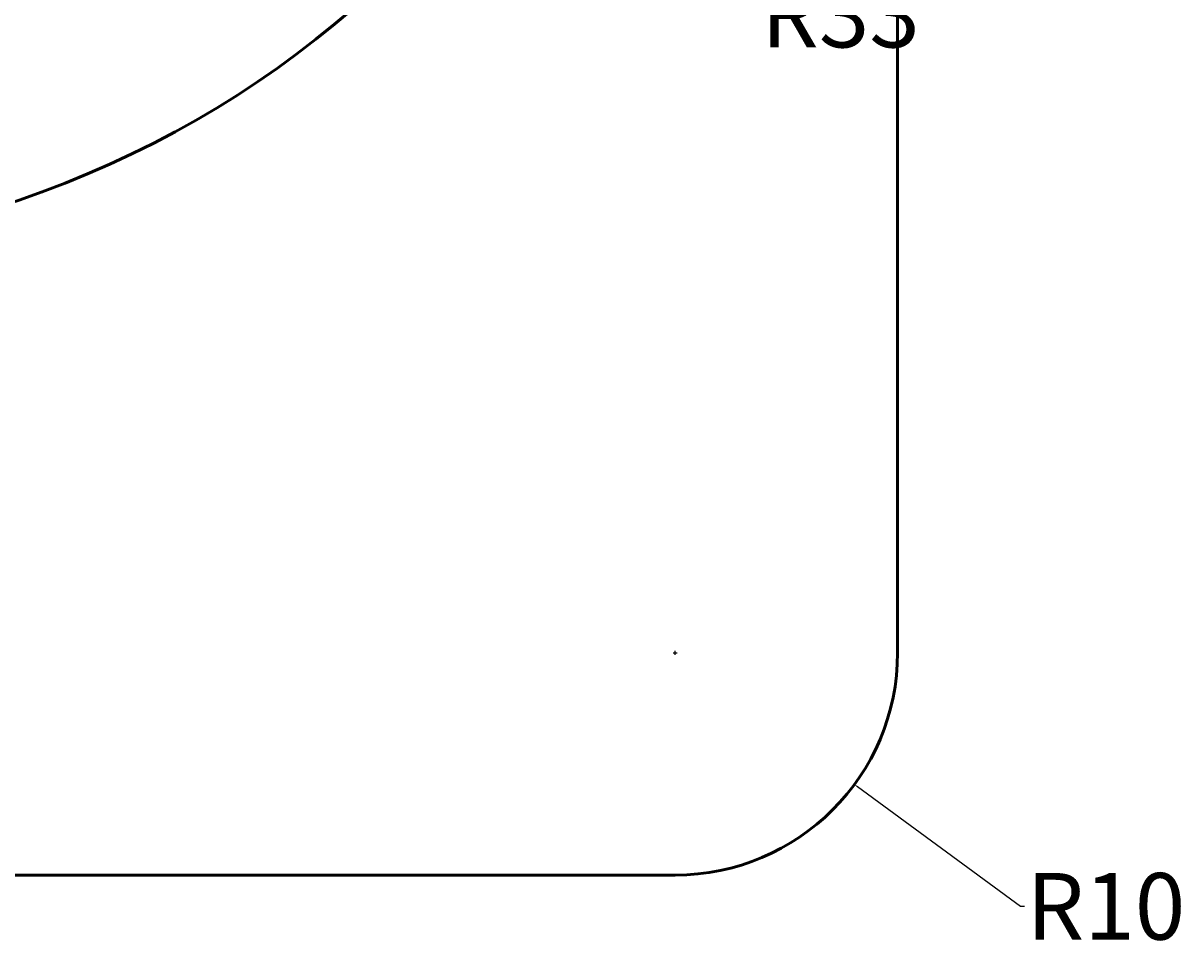
# Model space of a CAD drawing. Units: millimetres. Extents: x -50 to 109, y -46 to 152.
# Tile 9 of 18: x 48 to 100, y -10 to 32. Entities that reach past the tile are written whole.
import ezdxf

# ---------------------------------------------------------------- set-up
doc = ezdxf.new("R2010")
doc.units = ezdxf.units.MM
doc.header["$MEASUREMENT"] = 0
doc.layers.add('M-DIMS', color=2, linetype='Continuous', lineweight=25)
doc.layers.add('M-OUTL', color=7, linetype='Continuous', lineweight=50)
doc.styles.get("Standard").update_dxf_attribs({"font": 'arial.ttf'})
doc.dimstyles.get("Standard").update_dxf_attribs({"dimtxt": 0.18, "dimasz": 0.18, "dimexe": 0.18, "dimexo": 0.0625, "dimgap": 0.09, "dimtad": 0, "dimtih": 1, "dimtoh": 1, "dimdec": 4, "dimzin": 0, "dimdsep": 46, "dimtxsty": 'Standard', "dimcen": 0.09, "dimadec": 0, "dimazin": 0, "dimtfac": 1, "dimtdec": 4, "dimtofl": 0, "dimtmove": 0, "dimatfit": 3, "dimfxl": 1, "dimtolj": 1, "dimtzin": 0, "dimarcsym": 0})

# ---------------------------------------------------------------- blocks, each defined once
blk = doc.blocks.new('*D18')
at = {"layer": 'Defpoints', "color": 0, "transparency": 16777216}
for p in [(33.131, 66.25), (59.909, 46.965)]:
    blk.add_point(p, dxfattribs=at)
at = {"layer": 'M-DIMS', "color": 0, "lineweight": -2, "transparency": 16777216}
for p, q in [((33.041, 66.25), (33.221, 66.25)), ((33.131, 66.16), (33.131, 66.34)), ((80.717, 31.98), (60.055, 46.86)), ((80.897, 31.98), (80.717, 31.98))]:
    blk.add_line(p, q, dxfattribs=at)
at = {"layer": 'M-DIMS', "color": 0, "transparency": 16777216}
blk.add_solid([(60.073, 46.884), (60.038, 46.835), (59.909, 46.965)], dxfattribs=at)
at = {"layer": 'M-DIMS', "color": 0, "transparency": 16777216, "insert": (84.571, 31.98), "char_height": 0.18, "attachment_point": 5}
blk.add_mtext('\\A1;{\\H16.66667x;R33}', dxfattribs=at)
blk = doc.blocks.new('*D26')
at = {"layer": 'Defpoints', "color": 0, "transparency": 16777216}
for p in [(77.14, 3.241), (85.198, -2.681)]:
    blk.add_point(p, dxfattribs=at)
at = {"layer": 'M-DIMS', "color": 0, "lineweight": -2, "transparency": 16777216}
for p, q in [((77.05, 3.241), (77.23, 3.241)), ((77.14, 3.151), (77.14, 3.331)), ((92.661, -8.165), (85.343, -2.787)), ((92.841, -8.165), (92.661, -8.165))]:
    blk.add_line(p, q, dxfattribs=at)
at = {"layer": 'M-DIMS', "color": 0, "transparency": 16777216}
blk.add_solid([(85.361, -2.763), (85.326, -2.812), (85.198, -2.681)], dxfattribs=at)
at = {"layer": 'M-DIMS', "color": 0, "transparency": 16777216, "insert": (96.51, -8.165), "char_height": 0.18, "attachment_point": 5}
blk.add_mtext('\\A1;{\\H16.66667x;R10}', dxfattribs=at)

msp = doc.modelspace()

# ---------------------------------------------------------------- linework, layer by layer
at = {"layer": 'M-OUTL'}
for p, q in [((87.14026, 66.21184), (87.14026, 3.24112)), ((77.14026, -6.75888), (43.62689, -6.75888)), ((71.14503, -6.75826), (71.14503, -6.75888))]:
    msp.add_line(p, q, dxfattribs=at)
for centre, radius, start, end in [((33.197, 66.24997), 45, 180.010473, 359.989527), ((77.14026, 3.24112), 10, 270, 0)]:
    msp.add_arc(centre, radius, start, end, dxfattribs=at)

# ---------------------------------------------------------------- dimensions: what is measured, and where the dimension line sits
at = {"layer": 'M-DIMS'}
for center, mpoint, text, picture, middle in [((33.1307, 66.24997), (59.90911, 46.96483), '{\\H16.66667x;R33}', '*D18', (84.57118, 31.97955)), ((77.14026, 3.24112), (85.19823, -2.6808), '{\\H16.66667x;R10}', '*D26', (96.50965, -8.16494))]:
    dim = msp.add_radius_dim(center=center, mpoint=mpoint, text=text, dimstyle='Standard', override={"dimclrd": 0, "dimclre": 0, "dimclrt": 0}, dxfattribs=at)
    dim.commit()
    dim.dimension.update_dxf_attribs({"geometry": picture, "text_midpoint": middle, "dimtype": 164})

doc.saveas('drawing.dxf')
